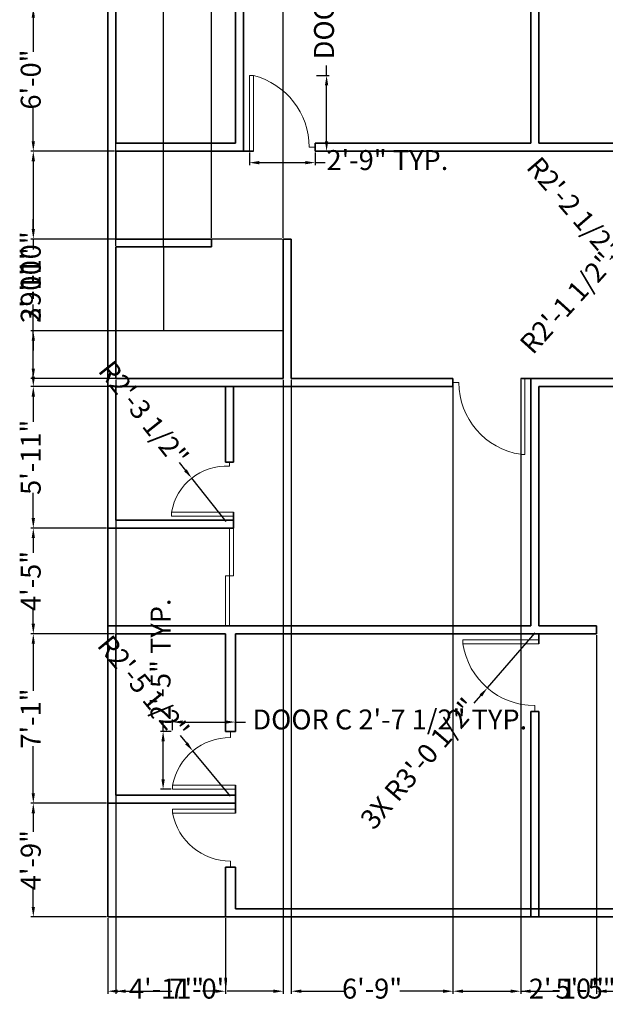
# Model space of a CAD drawing. Units: inches. Extents: x 2565 to 3182, y 2168 to 2957.
# Tile 1 of 3: x 2573 to 2867, y 2168 to 2662. Entities that reach past the tile are written whole.
import ezdxf

# ---------------------------------------------------------------- set-up
doc = ezdxf.new("R2010")
doc.units = ezdxf.units.IN
for name, color, linetype, lineweight in [('A-ANNO-DIMS', 2, 'Continuous', 13), ('A-DOOR', 4, 'Continuous', 18), ('A-FLOR-FIXT', 9, 'Continuous', 25), ('A-GLAZ', 3, 'Continuous', 18), ('A-WALL', 7, 'Continuous', 35)]:
    doc.layers.add(name, color=color, linetype=linetype, lineweight=lineweight)
doc.styles.get("Standard").update_dxf_attribs({"font": 'arial.ttf'})
doc.dimstyles.new('ISO-25', dxfattribs={"dimtxt": 10, "dimasz": 5, "dimexe": 1.25, "dimexo": 0.625, "dimtad": 0, "dimdec": 0, "dimrnd": 10, "dimlunit": 3, "dimtxsty": 'Standard', "dimcen": 2.5, "dimadec": 0, "dimazin": 0, "dimtfac": 1, "dimtdec": 0, "dimtmove": 0, "dimatfit": 3, "dimfxl": 1, "dimarcsym": 0})

# ---------------------------------------------------------------- blocks, each defined once
blk = doc.blocks.new('DOOR-SWING-36-OPENING-39')
for p, q in [((2, 36), (2, 33)), ((38, 2), (0, 2)), ((0, 2), (0, 0)), ((2, 0), (38, 0)), ((38, 0), (38, 2))]:
    blk.add_line(p, q)
blk.add_arc((2, -3.4), 36.4, 8.5358, 90)
blk = doc.blocks.new('DOOR-SWING-36-OPENING-36')
for p, q in [((0, 2), (0, 38)), ((0, 38), (2, 38)), ((2, 38), (2, 0)), ((0, 0), (0, 2)), ((33, 2), (30, 2)), ((2, 0), (0, 0))]:
    blk.add_line(p, q)
blk.add_arc((-7.14, 2), 37.14, 0, 75.75)
blk = doc.blocks.new('DOOR-SWING-29-OPENING-32')
for p, q in [((29, 29), (29, 26)), ((0, 0), (0, 2)), ((0, 2), (31.5, 2)), ((29, 0), (0, 0)), ((31.5, 2), (31.5, 0))]:
    blk.add_line(p, q)
blk.add_arc((29, -3.52), 29.52, 90, 169.2214)
blk = doc.blocks.new('*D9')
at = {"layer": 'A-ANNO-DIMS', "color": 0, "lineweight": -2, "transparency": 16777216}
for p, q in [((2727.13, 2633.77), (2727.13, 2638.77)), ((2722.05, 2633.77), (2728.38, 2633.77)), ((2727.13, 2600.77), (2727.13, 2628.77)), ((2722.05, 2595.77), (2728.38, 2595.77))]:
    blk.add_line(p, q, dxfattribs=at)
at = {"layer": 'A-ANNO-DIMS', "color": 0, "transparency": 16777216}
for points in [[(2726.3, 2628.77), (2727.96, 2628.77), (2727.13, 2633.77)], [(2726.3, 2600.77), (2727.96, 2600.77), (2727.13, 2595.77)]]:
    blk.add_solid(points, dxfattribs=at)
at = {"layer": 'Defpoints', "color": 0, "transparency": 16777216}
for p in [(2721.43, 2633.77), (2727.13, 2633.77), (2721.43, 2595.77)]:
    blk.add_point(p, dxfattribs=at)
at = {"layer": 'A-ANNO-DIMS', "color": 0, "transparency": 16777216, "insert": (2727.13, 2699.12), "char_height": 10, "attachment_point": 5, "rotation": 90}
blk.add_mtext('DOOR B 3\'-2" TYP.', dxfattribs=at)
blk = doc.blocks.new('*D10')
at = {"layer": 'A-ANNO-DIMS', "color": 0, "lineweight": -2, "transparency": 16777216}
for p, q in [((2688.43, 2595.14), (2688.43, 2588.82)), ((2721.43, 2595.14), (2721.43, 2588.82)), ((2693.43, 2590.07), (2716.43, 2590.07)), ((2721.43, 2590.07), (2726.43, 2590.07))]:
    blk.add_line(p, q, dxfattribs=at)
at = {"layer": 'A-ANNO-DIMS', "color": 0, "transparency": 16777216}
for points in [[(2693.43, 2590.9), (2693.43, 2589.23), (2688.43, 2590.07)], [(2716.43, 2590.9), (2716.43, 2589.23), (2721.43, 2590.07)]]:
    blk.add_solid(points, dxfattribs=at)
at = {"layer": 'Defpoints', "color": 0, "transparency": 16777216}
for p in [(2688.43, 2595.77), (2721.43, 2595.77), (2721.43, 2590.07)]:
    blk.add_point(p, dxfattribs=at)
at = {"layer": 'A-ANNO-DIMS', "color": 0, "transparency": 16777216, "insert": (2757.62, 2590.07), "char_height": 10, "attachment_point": 5}
blk.add_mtext('2\'-9" TYP.', dxfattribs=at)
blk = doc.blocks.new('*D11')
at = {"layer": 'A-ANNO-DIMS', "color": 0, "lineweight": -2, "transparency": 16777216}
for p, q in [((2649.93, 2305.39), (2649.93, 2310.74)), ((2654.93, 2309.49), (2676.43, 2309.49)), ((2681.43, 2305.39), (2681.43, 2310.74)), ((2681.43, 2309.49), (2686.43, 2309.49))]:
    blk.add_line(p, q, dxfattribs=at)
at = {"layer": 'A-ANNO-DIMS', "color": 0, "transparency": 16777216}
for points in [[(2654.93, 2310.33), (2654.93, 2308.66), (2649.93, 2309.49)], [(2676.43, 2310.33), (2676.43, 2308.66), (2681.43, 2309.49)]]:
    blk.add_solid(points, dxfattribs=at)
at = {"layer": 'Defpoints', "color": 0, "transparency": 16777216}
for p in [(2681.43, 2309.49), (2649.93, 2304.77), (2681.43, 2304.77)]:
    blk.add_point(p, dxfattribs=at)
at = {"layer": 'A-ANNO-DIMS', "color": 0, "transparency": 16777216, "insert": (2758.81, 2309.49), "char_height": 10, "attachment_point": 5}
blk.add_mtext('DOOR C 2\'-7 1/2" TYP.', dxfattribs=at)
blk = doc.blocks.new('*D12')
at = {"layer": 'A-ANNO-DIMS', "color": 0, "lineweight": -2, "transparency": 16777216}
for p, q in [((2645.2, 2304.77), (2645.2, 2309.77)), ((2649.3, 2304.77), (2643.95, 2304.77)), ((2645.2, 2280.77), (2645.2, 2299.77)), ((2649.3, 2275.77), (2643.95, 2275.77))]:
    blk.add_line(p, q, dxfattribs=at)
at = {"layer": 'A-ANNO-DIMS', "color": 0, "transparency": 16777216}
for points in [[(2644.37, 2299.77), (2646.04, 2299.77), (2645.2, 2304.77)], [(2644.37, 2280.77), (2646.04, 2280.77), (2645.2, 2275.77)]]:
    blk.add_solid(points, dxfattribs=at)
at = {"layer": 'Defpoints', "color": 0, "transparency": 16777216}
for p in [(2645.2, 2304.77), (2649.93, 2304.77), (2649.93, 2275.77)]:
    blk.add_point(p, dxfattribs=at)
at = {"layer": 'A-ANNO-DIMS', "color": 0, "transparency": 16777216, "insert": (2645.2, 2340.96), "char_height": 10, "attachment_point": 5, "rotation": 90}
blk.add_mtext('2\'-5" TYP.', dxfattribs=at)
blk = doc.blocks.new('*D18')
at = {"layer": 'A-ANNO-DIMS', "color": 0, "lineweight": -2, "transparency": 16777216}
for p, q in [((2616.8, 2268.77), (2578.9, 2268.77)), ((2580.15, 2263.77), (2580.15, 2254.39)), ((2580.15, 2216.77), (2580.15, 2226.15)), ((2616.8, 2211.77), (2578.9, 2211.77))]:
    blk.add_line(p, q, dxfattribs=at)
at = {"layer": 'A-ANNO-DIMS', "color": 0, "transparency": 16777216}
for points in [[(2579.32, 2263.77), (2580.98, 2263.77), (2580.15, 2268.77)], [(2579.32, 2216.77), (2580.98, 2216.77), (2580.15, 2211.77)]]:
    blk.add_solid(points, dxfattribs=at)
at = {"layer": 'Defpoints', "color": 0, "transparency": 16777216}
for p in [(2580.15, 2268.77), (2617.43, 2268.77), (2617.43, 2211.77)]:
    blk.add_point(p, dxfattribs=at)
at = {"layer": 'A-ANNO-DIMS', "color": 0, "transparency": 16777216, "insert": (2580.15, 2240.27), "char_height": 10, "attachment_point": 5, "rotation": 90}
blk.add_mtext('4\'-9"', dxfattribs=at)
blk = doc.blocks.new('*D19')
at = {"layer": 'A-ANNO-DIMS', "color": 0, "lineweight": -2, "transparency": 16777216}
for p, q in [((2620.8, 2353.77), (2578.9, 2353.77)), ((2580.15, 2348.77), (2580.15, 2325.14)), ((2580.15, 2273.77), (2580.15, 2297.39)), ((2616.8, 2268.77), (2578.9, 2268.77))]:
    blk.add_line(p, q, dxfattribs=at)
at = {"layer": 'A-ANNO-DIMS', "color": 0, "transparency": 16777216}
for points in [[(2579.32, 2348.77), (2580.98, 2348.77), (2580.15, 2353.77)], [(2579.32, 2273.77), (2580.98, 2273.77), (2580.15, 2268.77)]]:
    blk.add_solid(points, dxfattribs=at)
at = {"layer": 'Defpoints', "color": 0, "transparency": 16777216}
for p in [(2580.15, 2353.77), (2621.43, 2353.77), (2617.43, 2268.77)]:
    blk.add_point(p, dxfattribs=at)
at = {"layer": 'A-ANNO-DIMS', "color": 0, "transparency": 16777216, "insert": (2580.15, 2311.27), "char_height": 10, "attachment_point": 5, "rotation": 90}
blk.add_mtext('7\'-1"', dxfattribs=at)
blk = doc.blocks.new('*D20')
at = {"layer": 'A-ANNO-DIMS', "color": 0, "lineweight": -2, "transparency": 16777216}
for p, q in [((2616.8, 2406.77), (2578.9, 2406.77)), ((2580.15, 2401.77), (2580.15, 2394.39)), ((2580.15, 2358.77), (2580.15, 2366.15)), ((2620.8, 2353.77), (2578.9, 2353.77))]:
    blk.add_line(p, q, dxfattribs=at)
at = {"layer": 'A-ANNO-DIMS', "color": 0, "transparency": 16777216}
for points in [[(2579.32, 2401.77), (2580.98, 2401.77), (2580.15, 2406.77)], [(2579.32, 2358.77), (2580.98, 2358.77), (2580.15, 2353.77)]]:
    blk.add_solid(points, dxfattribs=at)
at = {"layer": 'Defpoints', "color": 0, "transparency": 16777216}
for p in [(2580.15, 2406.77), (2617.43, 2406.77), (2621.43, 2353.77)]:
    blk.add_point(p, dxfattribs=at)
at = {"layer": 'A-ANNO-DIMS', "color": 0, "transparency": 16777216, "insert": (2580.15, 2380.27), "char_height": 10, "attachment_point": 5, "rotation": 90}
blk.add_mtext('4\'-5"', dxfattribs=at)
blk = doc.blocks.new('*D21')
at = {"layer": 'A-ANNO-DIMS', "color": 0, "lineweight": -2, "transparency": 16777216}
for p, q in [((2620.8, 2477.77), (2578.9, 2477.77)), ((2580.15, 2472.77), (2580.15, 2460.07)), ((2580.15, 2411.77), (2580.15, 2424.47)), ((2616.8, 2406.77), (2578.9, 2406.77))]:
    blk.add_line(p, q, dxfattribs=at)
at = {"layer": 'A-ANNO-DIMS', "color": 0, "transparency": 16777216}
for points in [[(2579.32, 2472.77), (2580.98, 2472.77), (2580.15, 2477.77)], [(2579.32, 2411.77), (2580.98, 2411.77), (2580.15, 2406.77)]]:
    blk.add_solid(points, dxfattribs=at)
at = {"layer": 'Defpoints', "color": 0, "transparency": 16777216}
for p in [(2580.15, 2477.77), (2621.43, 2477.77), (2617.43, 2406.77)]:
    blk.add_point(p, dxfattribs=at)
at = {"layer": 'A-ANNO-DIMS', "color": 0, "transparency": 16777216, "insert": (2580.15, 2442.27), "char_height": 10, "attachment_point": 5, "rotation": 90}
blk.add_mtext('5\'-11"', dxfattribs=at)
blk = doc.blocks.new('*D22')
at = {"layer": 'A-ANNO-DIMS', "color": 0, "lineweight": -2, "transparency": 16777216}
for p, q in [((2620.8, 2595.77), (2578.9, 2595.77)), ((2580.15, 2590.77), (2580.15, 2554.57)), ((2580.15, 2482.77), (2580.15, 2518.97)), ((2620.8, 2477.77), (2578.9, 2477.77))]:
    blk.add_line(p, q, dxfattribs=at)
at = {"layer": 'A-ANNO-DIMS', "color": 0, "transparency": 16777216}
for points in [[(2579.32, 2590.77), (2580.98, 2590.77), (2580.15, 2595.77)], [(2579.32, 2482.77), (2580.98, 2482.77), (2580.15, 2477.77)]]:
    blk.add_solid(points, dxfattribs=at)
at = {"layer": 'Defpoints', "color": 0, "transparency": 16777216}
for p in [(2580.15, 2595.77), (2621.43, 2595.77), (2621.43, 2477.77)]:
    blk.add_point(p, dxfattribs=at)
at = {"layer": 'A-ANNO-DIMS', "color": 0, "transparency": 16777216, "insert": (2580.15, 2536.77), "char_height": 10, "attachment_point": 5, "rotation": 90}
blk.add_mtext('9\'-10"', dxfattribs=at)
blk = doc.blocks.new('*D23')
at = {"layer": 'A-ANNO-DIMS', "color": 0, "lineweight": -2, "transparency": 16777216}
for p, q in [((2620.8, 2667.77), (2578.9, 2667.77)), ((2580.15, 2662.77), (2580.15, 2645.71)), ((2580.15, 2600.77), (2580.15, 2617.82)), ((2620.8, 2595.77), (2578.9, 2595.77))]:
    blk.add_line(p, q, dxfattribs=at)
at = {"layer": 'A-ANNO-DIMS', "color": 0, "transparency": 16777216}
for points in [[(2579.32, 2662.77), (2580.98, 2662.77), (2580.15, 2667.77)], [(2579.32, 2600.77), (2580.98, 2600.77), (2580.15, 2595.77)]]:
    blk.add_solid(points, dxfattribs=at)
at = {"layer": 'Defpoints', "color": 0, "transparency": 16777216}
for p in [(2580.15, 2667.77), (2621.43, 2667.77), (2621.43, 2595.77)]:
    blk.add_point(p, dxfattribs=at)
at = {"layer": 'A-ANNO-DIMS', "color": 0, "transparency": 16777216, "insert": (2580.15, 2631.77), "char_height": 10, "attachment_point": 5, "rotation": 90}
blk.add_mtext('6\'-0"', dxfattribs=at)
blk = doc.blocks.new('*D36')
at = {"layer": 'A-ANNO-DIMS', "color": 0, "lineweight": -2, "transparency": 16777216}
for p, q in [((2617.43, 2211.14), (2617.43, 2173.24)), ((2676.43, 2211.14), (2676.43, 2173.24)), ((2622.43, 2174.49), (2628.93, 2174.49)), ((2671.43, 2174.49), (2664.93, 2174.49))]:
    blk.add_line(p, q, dxfattribs=at)
at = {"layer": 'A-ANNO-DIMS', "color": 0, "transparency": 16777216}
for points in [[(2622.43, 2175.32), (2622.43, 2173.65), (2617.43, 2174.49)], [(2671.43, 2175.32), (2671.43, 2173.65), (2676.43, 2174.49)]]:
    blk.add_solid(points, dxfattribs=at)
at = {"layer": 'Defpoints', "color": 0, "transparency": 16777216}
for p in [(2617.43, 2211.77), (2676.43, 2211.77), (2676.43, 2174.49)]:
    blk.add_point(p, dxfattribs=at)
at = {"layer": 'A-ANNO-DIMS', "color": 0, "transparency": 16777216, "insert": (2646.93, 2174.49), "char_height": 10, "attachment_point": 5}
blk.add_mtext('4\'-11"', dxfattribs=at)
blk = doc.blocks.new('*D38')
at = {"layer": 'A-ANNO-DIMS', "color": 0, "lineweight": -2, "transparency": 16777216}
for p, q in [((2862.43, 2353.14), (2862.43, 2173.24)), ((2924.43, 2353.14), (2924.43, 2173.24)), ((2867.43, 2174.49), (2879.51, 2174.49)), ((2919.43, 2174.49), (2907.35, 2174.49))]:
    blk.add_line(p, q, dxfattribs=at)
at = {"layer": 'A-ANNO-DIMS', "color": 0, "transparency": 16777216}
for points in [[(2867.43, 2175.32), (2867.43, 2173.65), (2862.43, 2174.49)], [(2919.43, 2175.32), (2919.43, 2173.65), (2924.43, 2174.49)]]:
    blk.add_solid(points, dxfattribs=at)
at = {"layer": 'Defpoints', "color": 0, "transparency": 16777216}
for p in [(2862.43, 2353.77), (2924.43, 2353.77), (2924.43, 2174.49)]:
    blk.add_point(p, dxfattribs=at)
at = {"layer": 'A-ANNO-DIMS', "color": 0, "transparency": 16777216, "insert": (2893.43, 2174.49), "char_height": 10, "attachment_point": 5}
blk.add_mtext('5\'-2"', dxfattribs=at)
blk = doc.blocks.new('*D39')
at = {"layer": 'A-ANNO-DIMS', "color": 0, "lineweight": -2, "transparency": 16777216}
for p, q in [((2621.43, 2481.14), (2621.43, 2173.24)), ((2705.43, 2481.14), (2705.43, 2173.24)), ((2626.43, 2174.49), (2649.55, 2174.49)), ((2700.43, 2174.49), (2677.3, 2174.49))]:
    blk.add_line(p, q, dxfattribs=at)
at = {"layer": 'A-ANNO-DIMS', "color": 0, "transparency": 16777216}
for points in [[(2626.43, 2175.32), (2626.43, 2173.65), (2621.43, 2174.49)], [(2700.43, 2175.32), (2700.43, 2173.65), (2705.43, 2174.49)]]:
    blk.add_solid(points, dxfattribs=at)
at = {"layer": 'Defpoints', "color": 0, "transparency": 16777216}
for p in [(2621.43, 2481.77), (2705.43, 2481.77), (2705.43, 2174.49)]:
    blk.add_point(p, dxfattribs=at)
at = {"layer": 'A-ANNO-DIMS', "color": 0, "transparency": 16777216, "insert": (2663.43, 2174.49), "char_height": 10, "attachment_point": 5}
blk.add_mtext('7\'-0"', dxfattribs=at)
blk = doc.blocks.new('*D40')
at = {"layer": 'A-ANNO-DIMS', "color": 0, "lineweight": -2, "transparency": 16777216}
for p, q in [((2709.43, 2481.14), (2709.43, 2173.24)), ((2790.43, 2481.14), (2790.43, 2173.24)), ((2714.43, 2174.49), (2735.99, 2174.49)), ((2785.43, 2174.49), (2763.87, 2174.49))]:
    blk.add_line(p, q, dxfattribs=at)
at = {"layer": 'A-ANNO-DIMS', "color": 0, "transparency": 16777216}
for points in [[(2714.43, 2175.32), (2714.43, 2173.65), (2709.43, 2174.49)], [(2785.43, 2175.32), (2785.43, 2173.65), (2790.43, 2174.49)]]:
    blk.add_solid(points, dxfattribs=at)
at = {"layer": 'Defpoints', "color": 0, "transparency": 16777216}
for p in [(2709.43, 2481.77), (2790.43, 2481.77), (2790.43, 2174.49)]:
    blk.add_point(p, dxfattribs=at)
at = {"layer": 'A-ANNO-DIMS', "color": 0, "transparency": 16777216, "insert": (2749.93, 2174.49), "char_height": 10, "attachment_point": 5}
blk.add_mtext('6\'-9"', dxfattribs=at)
blk = doc.blocks.new('*D41')
at = {"layer": 'A-ANNO-DIMS', "color": 0, "lineweight": -2, "transparency": 16777216}
for p, q in [((2580.15, 2556.77), (2580.15, 2561.77)), ((2704.8, 2551.77), (2578.9, 2551.77)), ((2580.15, 2551.77), (2580.15, 2546.57)), ((2580.15, 2505.77), (2580.15, 2510.97)), ((2704.8, 2505.77), (2578.9, 2505.77)), ((2580.15, 2500.77), (2580.15, 2495.77))]:
    blk.add_line(p, q, dxfattribs=at)
at = {"layer": 'A-ANNO-DIMS', "color": 0, "transparency": 16777216}
for points in [[(2579.32, 2556.77), (2580.98, 2556.77), (2580.15, 2551.77)], [(2579.32, 2500.77), (2580.98, 2500.77), (2580.15, 2505.77)]]:
    blk.add_solid(points, dxfattribs=at)
at = {"layer": 'Defpoints', "color": 0, "transparency": 16777216}
for p in [(2580.15, 2551.77), (2705.43, 2551.77), (2705.43, 2505.77)]:
    blk.add_point(p, dxfattribs=at)
at = {"layer": 'A-ANNO-DIMS', "color": 0, "transparency": 16777216, "insert": (2580.15, 2528.77), "char_height": 10, "attachment_point": 5, "rotation": 90}
blk.add_mtext('3\'-10"', dxfattribs=at)
blk = doc.blocks.new('*D42')
at = {"layer": 'A-ANNO-DIMS', "color": 0, "lineweight": -2, "transparency": 16777216}
for p, q in [((2664.43, 2897.05), (2659.43, 2897.05)), ((2669.43, 2552.39), (2669.43, 2898.3)), ((2669.43, 2897.05), (2673.52, 2897.05)), ((2705.43, 2897.05), (2701.34, 2897.05)), ((2705.43, 2552.39), (2705.43, 2898.3)), ((2710.43, 2897.05), (2715.43, 2897.05))]:
    blk.add_line(p, q, dxfattribs=at)
at = {"layer": 'A-ANNO-DIMS', "color": 0, "transparency": 16777216}
for points in [[(2664.43, 2897.88), (2664.43, 2896.21), (2669.43, 2897.05)], [(2710.43, 2897.88), (2710.43, 2896.21), (2705.43, 2897.05)]]:
    blk.add_solid(points, dxfattribs=at)
at = {"layer": 'Defpoints', "color": 0, "transparency": 16777216}
for p in [(2705.43, 2897.05), (2669.43, 2551.77), (2705.43, 2551.77)]:
    blk.add_point(p, dxfattribs=at)
at = {"layer": 'A-ANNO-DIMS', "color": 0, "transparency": 16777216, "insert": (2687.43, 2897.05), "char_height": 10, "attachment_point": 5}
blk.add_mtext('3\'-0"', dxfattribs=at)
blk = doc.blocks.new('*D43')
at = {"layer": 'A-ANNO-DIMS', "color": 0, "lineweight": -2, "transparency": 16777216}
for p, q in [((2621.43, 2548.39), (2621.43, 2898.3)), ((2626.43, 2897.05), (2640.43, 2897.05)), ((2645.43, 2548.39), (2645.43, 2898.3)), ((2645.43, 2897.05), (2650.43, 2897.05))]:
    blk.add_line(p, q, dxfattribs=at)
at = {"layer": 'A-ANNO-DIMS', "color": 0, "transparency": 16777216}
for points in [[(2626.43, 2897.88), (2626.43, 2896.21), (2621.43, 2897.05)], [(2640.43, 2897.88), (2640.43, 2896.21), (2645.43, 2897.05)]]:
    blk.add_solid(points, dxfattribs=at)
at = {"layer": 'Defpoints', "color": 0, "transparency": 16777216}
for p in [(2645.43, 2897.05), (2621.43, 2547.77), (2645.43, 2547.77)]:
    blk.add_point(p, dxfattribs=at)
at = {"layer": 'A-ANNO-DIMS', "color": 0, "transparency": 16777216, "insert": (2664.43, 2897.05), "char_height": 10, "attachment_point": 5}
blk.add_mtext('2\'-0"', dxfattribs=at)
blk = doc.blocks.new('*D44')
at = {"layer": 'A-ANNO-DIMS', "color": 0, "lineweight": -2, "transparency": 16777216}
for p, q in [((2580.15, 2505.77), (2580.15, 2510.77)), ((2704.8, 2505.77), (2578.9, 2505.77)), ((2580.15, 2486.77), (2580.15, 2500.77)), ((2704.8, 2481.77), (2578.9, 2481.77))]:
    blk.add_line(p, q, dxfattribs=at)
at = {"layer": 'A-ANNO-DIMS', "color": 0, "transparency": 16777216}
for points in [[(2579.32, 2500.77), (2580.98, 2500.77), (2580.15, 2505.77)], [(2579.32, 2486.77), (2580.98, 2486.77), (2580.15, 2481.77)]]:
    blk.add_solid(points, dxfattribs=at)
at = {"layer": 'Defpoints', "color": 0, "transparency": 16777216}
for p in [(2580.15, 2505.77), (2705.43, 2505.77), (2705.43, 2481.77)]:
    blk.add_point(p, dxfattribs=at)
at = {"layer": 'A-ANNO-DIMS', "color": 0, "transparency": 16777216, "insert": (2580.15, 2524.77), "char_height": 10, "attachment_point": 5, "rotation": 90}
blk.add_mtext('2\'-0"', dxfattribs=at)
blk = doc.blocks.new('*D47')
at = {"layer": 'A-ANNO-DIMS', "color": 0, "lineweight": -2, "transparency": 16777216}
for p, q in [((2790.43, 2481.14), (2790.43, 2173.24)), ((2824.43, 2481.14), (2824.43, 2173.24)), ((2795.43, 2174.49), (2819.43, 2174.49)), ((2824.43, 2174.49), (2829.43, 2174.49))]:
    blk.add_line(p, q, dxfattribs=at)
at = {"layer": 'A-ANNO-DIMS', "color": 0, "transparency": 16777216}
for points in [[(2795.43, 2175.32), (2795.43, 2173.65), (2790.43, 2174.49)], [(2819.43, 2175.32), (2819.43, 2173.65), (2824.43, 2174.49)]]:
    blk.add_solid(points, dxfattribs=at)
at = {"layer": 'Defpoints', "color": 0, "transparency": 16777216}
for p in [(2790.43, 2481.77), (2824.43, 2481.77), (2824.43, 2174.49)]:
    blk.add_point(p, dxfattribs=at)
at = {"layer": 'A-ANNO-DIMS', "color": 0, "transparency": 16777216, "insert": (2847.32, 2174.49), "char_height": 10, "attachment_point": 5}
blk.add_mtext('2\'-10"', dxfattribs=at)
blk = doc.blocks.new('*D48')
at = {"layer": 'A-ANNO-DIMS', "color": 0, "lineweight": -2, "transparency": 16777216}
for p, q in [((2824.43, 2481.14), (2824.43, 2173.24)), ((2889.43, 2481.14), (2889.43, 2173.24)), ((2829.43, 2174.49), (2843.01, 2174.49)), ((2884.43, 2174.49), (2870.85, 2174.49))]:
    blk.add_line(p, q, dxfattribs=at)
at = {"layer": 'A-ANNO-DIMS', "color": 0, "transparency": 16777216}
for points in [[(2829.43, 2175.32), (2829.43, 2173.65), (2824.43, 2174.49)], [(2884.43, 2175.32), (2884.43, 2173.65), (2889.43, 2174.49)]]:
    blk.add_solid(points, dxfattribs=at)
at = {"layer": 'Defpoints', "color": 0, "transparency": 16777216}
for p in [(2824.43, 2481.77), (2889.43, 2481.77), (2889.43, 2174.49)]:
    blk.add_point(p, dxfattribs=at)
at = {"layer": 'A-ANNO-DIMS', "color": 0, "transparency": 16777216, "insert": (2856.93, 2174.49), "char_height": 10, "attachment_point": 5}
blk.add_mtext('5\'-5"', dxfattribs=at)
blk = doc.blocks.new('*D63')
at = {"layer": 'A-ANNO-DIMS', "color": 0, "lineweight": -2, "transparency": 16777216}
for p, q in [((2831.43, 2354.17), (2807.68, 2326.59)), ((2801.15, 2319.01), (2804.41, 2322.8))]:
    blk.add_line(p, q, dxfattribs=at)
at = {"layer": 'A-ANNO-DIMS', "color": 0, "transparency": 16777216}
blk.add_solid([(2803.78, 2323.34), (2805.04, 2322.25), (2807.68, 2326.59)], dxfattribs=at)
at = {"layer": 'Defpoints', "color": 0, "transparency": 16777216}
for p in [(2831.43, 2354.17), (2807.68, 2326.59)]:
    blk.add_point(p, dxfattribs=at)
at = {"layer": 'A-ANNO-DIMS', "color": 0, "transparency": 16777216, "insert": (2774.34, 2287.87), "char_height": 10, "attachment_point": 5, "rotation": 49.2676}
blk.add_mtext('3X R3\'-0 1/2"', dxfattribs=at)
blk = doc.blocks.new('*D67')
at = {"layer": 'A-ANNO-DIMS', "color": 0, "lineweight": -2, "transparency": 16777216}
for p, q in [((2653.73, 2302.69), (2656.92, 2298.84)), ((2678.93, 2272.25), (2660.11, 2294.99))]:
    blk.add_line(p, q, dxfattribs=at)
at = {"layer": 'A-ANNO-DIMS', "color": 0, "transparency": 16777216}
blk.add_solid([(2657.56, 2299.37), (2656.28, 2298.31), (2660.11, 2294.99)], dxfattribs=at)
at = {"layer": 'Defpoints', "color": 0, "transparency": 16777216}
for p in [(2660.11, 2294.99), (2678.93, 2272.25)]:
    blk.add_point(p, dxfattribs=at)
at = {"layer": 'A-ANNO-DIMS', "color": 0, "transparency": 16777216, "insert": (2634.38, 2326.08), "char_height": 10, "attachment_point": 5, "rotation": 309.6098}
blk.add_mtext('R2\'-5 1/2"', dxfattribs=at)
blk = doc.blocks.new('*D68')
at = {"layer": 'A-ANNO-DIMS', "color": 0, "lineweight": -2, "transparency": 16777216}
for p, q in [((2653.31, 2439.66), (2656.41, 2435.74)), ((2676.72, 2410.14), (2659.52, 2431.83))]:
    blk.add_line(p, q, dxfattribs=at)
at = {"layer": 'A-ANNO-DIMS', "color": 0, "transparency": 16777216}
blk.add_solid([(2657.07, 2436.26), (2655.76, 2435.23), (2659.52, 2431.83)], dxfattribs=at)
at = {"layer": 'Defpoints', "color": 0, "transparency": 16777216}
for p in [(2659.52, 2431.83), (2676.72, 2410.14)]:
    blk.add_point(p, dxfattribs=at)
at = {"layer": 'A-ANNO-DIMS', "color": 0, "transparency": 16777216, "insert": (2634.45, 2463.44), "char_height": 10, "attachment_point": 5, "rotation": 308.4184}
blk.add_mtext('R2\'-3 1/2"', dxfattribs=at)
blk = doc.blocks.new('*D70')
at = {"layer": 'A-ANNO-DIMS', "color": 0, "lineweight": -2, "transparency": 16777216}
for p, q in [((2869.74, 2543.36), (2873.01, 2539.58)), ((2893.6, 2515.77), (2876.29, 2535.8))]:
    blk.add_line(p, q, dxfattribs=at)
at = {"layer": 'A-ANNO-DIMS', "color": 0, "transparency": 16777216}
blk.add_solid([(2873.65, 2540.13), (2872.38, 2539.04), (2876.29, 2535.8)], dxfattribs=at)
at = {"layer": 'Defpoints', "color": 0, "transparency": 16777216}
for p in [(2876.29, 2535.8), (2893.6, 2515.77)]:
    blk.add_point(p, dxfattribs=at)
at = {"layer": 'A-ANNO-DIMS', "color": 0, "transparency": 16777216, "insert": (2849.89, 2566.32), "char_height": 10, "attachment_point": 5, "rotation": 310.8471}
blk.add_mtext('R2\'-2 1/2"', dxfattribs=at)
blk = doc.blocks.new('*D72')
at = {"layer": 'A-ANNO-DIMS', "color": 0, "lineweight": -2, "transparency": 16777216}
for p, q in [((2892.82, 2567.71), (2875.74, 2548.82)), ((2869.03, 2541.41), (2872.38, 2545.11))]:
    blk.add_line(p, q, dxfattribs=at)
at = {"layer": 'A-ANNO-DIMS', "color": 0, "transparency": 16777216}
blk.add_solid([(2871.76, 2545.67), (2873, 2544.55), (2875.74, 2548.82)], dxfattribs=at)
at = {"layer": 'Defpoints', "color": 0, "transparency": 16777216}
for p in [(2892.82, 2567.71), (2875.74, 2548.82)]:
    blk.add_point(p, dxfattribs=at)
at = {"layer": 'A-ANNO-DIMS', "color": 0, "transparency": 16777216, "insert": (2848.67, 2518.9), "char_height": 10, "attachment_point": 5, "rotation": 47.8657}
blk.add_mtext('R2\'-1 1/2"', dxfattribs=at)

msp = doc.modelspace()

# ---------------------------------------------------------------- linework, layer by layer
at = {"layer": 'A-DOOR'}
for p, q in [((2826.43, 2481.77), (2826.43, 2479.77)), ((2678.43, 2439.77), (2678.43, 2437.77)), ((2649.43, 2412.77), (2649.43, 2414.77)), ((2649.43, 2414.77), (2680.43, 2414.77)), ((2678.43, 2412.77), (2649.43, 2412.77)), ((2680.43, 2412.77), (2678.43, 2412.77)), ((2680.43, 2414.77), (2680.43, 2412.77)), ((2680.43, 2412.77), (2680.43, 2412.77)), ((2833.43, 2350.77), (2829.43, 2350.77)), ((2678.93, 2275.77), (2678.93, 2275.77)), ((2681.43, 2275.77), (2678.93, 2275.77)), ((2681.43, 2265.77), (2677.72, 2265.77))]:
    msp.add_line(p, q, dxfattribs=at)
msp.add_arc((2676.72, 2410.14), 27.68, 86.4675, 170.3686, dxfattribs=at)
at = {"layer": 'A-FLOR-FIXT'}
for p in [(2645.43, 2547.77), (2705.43, 2505.77)]:
    msp.add_line(p, (2645.43, 2505.77), dxfattribs=at)
at = {"layer": 'A-GLAZ'}
for p, q in [((2678.43, 2382.77), (2678.43, 2406.77)), ((2680.43, 2406.77), (2680.43, 2382.77)), ((2676.43, 2357.77), (2676.43, 2382.77)), ((2676.43, 2382.77), (2678.43, 2382.77)), ((2680.43, 2382.77), (2678.43, 2382.77)), ((2678.43, 2382.77), (2678.43, 2357.77)), ((2678.43, 2357.77), (2676.43, 2357.77))]:
    msp.add_line(p, q, dxfattribs=at)
at = {"layer": 'A-WALL'}
for p, q in [((2617.43, 2859.77), (2617.43, 2211.77)), ((2829.43, 2719.77), (2829.43, 2599.77)), ((2833.43, 2719.77), (2833.43, 2599.77)), ((2685.43, 2671.77), (2685.43, 2595.77)), ((2621.43, 2667.77), (2621.43, 2599.77)), ((2681.43, 2667.77), (2681.43, 2599.77)), ((2681.43, 2599.77), (2621.43, 2599.77)), ((2685.43, 2599.77), (2685.43, 2595.77)), ((2721.43, 2599.77), (2721.43, 2595.77)), ((2829.43, 2599.77), (2721.43, 2599.77)), ((2893.43, 2599.77), (2833.43, 2599.77)), ((2690.43, 2595.77), (2621.43, 2595.77)), ((2621.43, 2595.77), (2621.43, 2551.77)), ((2889.43, 2595.77), (2721.43, 2595.77)), ((2669.43, 2551.77), (2621.43, 2551.77)), ((2669.43, 2547.77), (2669.43, 2551.77)), ((2709.43, 2551.77), (2705.43, 2551.77)), ((2705.43, 2549.77), (2705.43, 2551.77)), ((2705.43, 2545.77), (2705.43, 2549.77)), ((2709.43, 2551.77), (2709.43, 2481.77)), ((2669.43, 2547.77), (2621.43, 2547.77)), ((2621.43, 2547.77), (2621.43, 2481.77)), ((2705.43, 2547.77), (2705.43, 2481.77)), ((2705.43, 2481.77), (2621.43, 2481.77)), ((2790.43, 2481.77), (2709.43, 2481.77)), ((2790.43, 2477.77), (2790.43, 2481.77)), ((2889.43, 2481.77), (2824.43, 2481.77)), ((2829.43, 2477.77), (2829.43, 2481.77)), ((2681.43, 2477.77), (2621.43, 2477.77)), ((2621.43, 2477.77), (2621.43, 2421.77)), ((2676.43, 2477.77), (2676.43, 2439.77)), ((2680.43, 2477.77), (2680.43, 2439.77)), ((2681.43, 2477.77), (2685.43, 2477.77)), ((2790.43, 2477.77), (2685.43, 2477.77)), ((2829.43, 2477.77), (2829.43, 2357.77)), ((2893.43, 2477.77), (2833.43, 2477.77)), ((2833.43, 2477.77), (2833.43, 2357.77)), ((2676.43, 2439.77), (2680.43, 2439.77)), ((2621.43, 2421.77), (2621.43, 2410.77)), ((2676.43, 2410.77), (2621.43, 2410.77)), ((2676.43, 2410.77), (2680.43, 2410.77)), ((2680.43, 2406.77), (2680.43, 2414.77)), ((2621.43, 2406.77), (2617.43, 2406.77)), ((2680.43, 2406.77), (2621.43, 2406.77)), ((2621.43, 2406.77), (2621.43, 2406.77)), ((2676.43, 2406.77), (2680.43, 2406.77)), ((2621.43, 2357.77), (2617.43, 2357.77)), ((2681.43, 2357.77), (2621.43, 2357.77)), ((2685.43, 2357.77), (2681.43, 2357.77)), ((2829.43, 2357.77), (2685.43, 2357.77)), ((2862.43, 2357.77), (2833.43, 2357.77)), ((2862.43, 2353.77), (2862.43, 2357.77)), ((2676.43, 2353.77), (2621.43, 2353.77)), ((2621.43, 2353.77), (2621.43, 2272.77)), ((2676.43, 2353.77), (2676.43, 2304.77)), ((2681.43, 2353.77), (2681.43, 2304.77)), ((2685.43, 2353.77), (2681.43, 2353.77)), ((2829.43, 2353.77), (2685.43, 2353.77)), ((2829.43, 2353.77), (2833.43, 2353.77)), ((2833.43, 2353.77), (2833.43, 2348.77)), ((2862.43, 2353.77), (2833.43, 2353.77)), ((2829.43, 2314.77), (2833.43, 2314.77)), ((2829.43, 2314.77), (2829.43, 2211.77)), ((2833.43, 2314.77), (2833.43, 2211.77)), ((2676.43, 2304.77), (2681.43, 2304.77)), ((2681.43, 2277.77), (2681.43, 2263.77)), ((2621.43, 2272.77), (2676.43, 2272.77)), ((2676.43, 2272.77), (2681.43, 2272.77)), ((2621.43, 2268.77), (2617.43, 2268.77)), ((2621.43, 2268.77), (2676.43, 2268.77)), ((2676.43, 2268.77), (2681.43, 2268.77)), ((2676.43, 2236.77), (2681.43, 2236.77)), ((2676.43, 2236.77), (2676.43, 2215.77)), ((2681.43, 2236.77), (2681.43, 2215.77)), ((2676.43, 2215.77), (2676.43, 2211.77)), ((2681.43, 2215.77), (2953.43, 2215.77)), ((2617.43, 2211.77), (3093.43, 2211.77))]:
    msp.add_line(p, q, dxfattribs=at)

# ---------------------------------------------------------------- block references
at = {"layer": 'A-DOOR'}
for name, p in [('DOOR-SWING-36-OPENING-36', (2688.43, 2595.77)), ('DOOR-SWING-29-OPENING-32', (2649.93, 2275.77))]:
    msp.add_blockref(name, p, dxfattribs=at)
at = {"layer": 'A-DOOR', "extrusion": (0, 0, -1), "zscale": -1}
for name, p, rotation in [('DOOR-SWING-36-OPENING-39', (-2826.43, 2481.77), 269.9999999999969), ('DOOR-SWING-29-OPENING-32', (-2649.93, 2265.77), 180)]:
    msp.add_blockref(name, p, dxfattribs=dict(at, rotation=rotation))
at = {"layer": 'A-DOOR', "rotation": 180}
msp.add_blockref('DOOR-SWING-36-OPENING-39', (2833.43, 2350.77), dxfattribs=at)

# ---------------------------------------------------------------- dimensions: what is measured, and where the dimension line sits
at = {"layer": 'A-ANNO-DIMS'}
for base, p1, p2, picture, middle in [((2645.43, 2897.05), (2621.43, 2547.77), (2645.43, 2547.77), '*D43', (2664.43, 2897.05)), ((2705.43, 2897.05), (2669.43, 2551.77), (2705.43, 2551.77), '*D42', (2687.43, 2897.05)), ((2705.43, 2174.49), (2621.43, 2481.77), (2705.43, 2481.77), '*D39', (2663.43, 2174.49)), ((2790.43, 2174.49), (2709.43, 2481.77), (2790.43, 2481.77), '*D40', (2749.93, 2174.49)), ((2824.43, 2174.49), (2790.43, 2481.77), (2824.43, 2481.77), '*D47', (2847.32, 2174.49)), ((2889.43, 2174.49), (2824.43, 2481.77), (2889.43, 2481.77), '*D48', (2856.93, 2174.49)), ((2924.43, 2174.49), (2862.43, 2353.77), (2924.43, 2353.77), '*D38', (2893.43, 2174.49)), ((2676.43, 2174.49), (2617.43, 2211.77), (2676.43, 2211.77), '*D36', (2646.93, 2174.49))]:
    dim = msp.add_linear_dim(base=base, p1=p1, p2=p2, dimstyle='ISO-25', override={"dimdec": 1, "dimlfac": 1, "dimrnd": 0, "dimzin": 1, "dimdsep": 46, "dimlunit": 4, "dimfrac": 2}, dxfattribs=at)
    dim.commit()
    dim.dimension.update_dxf_attribs({"geometry": picture, "text_midpoint": middle})
for base, p1, p2, text, picture, middle in [((2727.13, 2633.77), (2721.43, 2595.77), (2721.43, 2633.77), 'DOOR B <> TYP.', '*D9', (2727.13, 2699.12)), ((2645.2, 2304.77), (2649.93, 2275.77), (2649.93, 2304.77), '<> TYP.', '*D12', (2645.2, 2340.96))]:
    dim = msp.add_linear_dim(base=base, p1=p1, p2=p2, angle=90, text=text, dimstyle='ISO-25', override={"dimdec": 1, "dimlfac": 1, "dimrnd": 0, "dimzin": 1, "dimdsep": 46, "dimlunit": 4, "dimfrac": 2}, dxfattribs=at)
    dim.commit()
    dim.dimension.update_dxf_attribs({"geometry": picture, "text_midpoint": middle})
for base, p1, p2, picture, middle in [((2580.15, 2667.77), (2621.43, 2595.77), (2621.43, 2667.77), '*D23', (2580.15, 2631.77)), ((2580.15, 2595.77), (2621.43, 2477.77), (2621.43, 2595.77), '*D22', (2580.15, 2536.77)), ((2580.15, 2551.77), (2705.43, 2505.77), (2705.43, 2551.77), '*D41', (2580.15, 2528.77)), ((2580.15, 2505.77), (2705.43, 2481.77), (2705.43, 2505.77), '*D44', (2580.15, 2524.77)), ((2580.15, 2477.77), (2617.43, 2406.77), (2621.43, 2477.77), '*D21', (2580.15, 2442.27)), ((2580.15, 2406.77), (2621.43, 2353.77), (2617.43, 2406.77), '*D20', (2580.15, 2380.27)), ((2580.15, 2353.77), (2617.43, 2268.77), (2621.43, 2353.77), '*D19', (2580.15, 2311.27)), ((2580.15, 2268.77), (2617.43, 2211.77), (2617.43, 2268.77), '*D18', (2580.15, 2240.27))]:
    dim = msp.add_linear_dim(base=base, p1=p1, p2=p2, angle=90, dimstyle='ISO-25', override={"dimdec": 1, "dimlfac": 1, "dimrnd": 0, "dimzin": 1, "dimdsep": 46, "dimlunit": 4, "dimfrac": 2}, dxfattribs=at)
    dim.commit()
    dim.dimension.update_dxf_attribs({"geometry": picture, "text_midpoint": middle})
for base, p1, p2, text, picture, middle in [((2721.43, 2590.07), (2688.43, 2595.77), (2721.43, 2595.77), '<> TYP.', '*D10', (2757.62, 2590.07)), ((2681.43, 2309.49), (2649.93, 2304.77), (2681.43, 2304.77), 'DOOR C <> TYP.', '*D11', (2758.81, 2309.49))]:
    dim = msp.add_linear_dim(base=base, p1=p1, p2=p2, text=text, dimstyle='ISO-25', override={"dimdec": 1, "dimlfac": 1, "dimrnd": 0, "dimzin": 1, "dimdsep": 46, "dimlunit": 4, "dimfrac": 2}, dxfattribs=at)
    dim.commit()
    dim.dimension.update_dxf_attribs({"geometry": picture, "text_midpoint": middle})
for center, mpoint, picture, middle in [((2893.6, 2515.77), (2876.29, 2535.8), '*D70', (2849.89, 2566.32)), ((2892.82, 2567.71), (2875.74, 2548.82), '*D72', (2848.67, 2518.9)), ((2676.72, 2410.14), (2659.52, 2431.83), '*D68', (2634.45, 2463.44)), ((2678.93, 2272.25), (2660.11, 2294.99), '*D67', (2634.38, 2326.08))]:
    dim = msp.add_radius_dim(center=center, mpoint=mpoint, dimstyle='ISO-25', override={"dimdec": 1, "dimlfac": 1, "dimrnd": 0, "dimzin": 1, "dimdsep": 46, "dimlunit": 4, "dimfrac": 2}, dxfattribs=at)
    dim.commit()
    dim.dimension.update_dxf_attribs({"geometry": picture, "text_midpoint": middle})
dim = msp.add_radius_dim(center=(2831.43, 2354.17), mpoint=(2807.68, 2326.59), text='3X <>', dimstyle='ISO-25', override={"dimdec": 1, "dimlfac": 1, "dimrnd": 0, "dimzin": 1, "dimdsep": 46, "dimlunit": 4, "dimfrac": 2}, dxfattribs=at)
dim.commit()
dim.dimension.update_dxf_attribs({"geometry": '*D63', "text_midpoint": (2774.34, 2287.87)})

doc.saveas('drawing.dxf')
